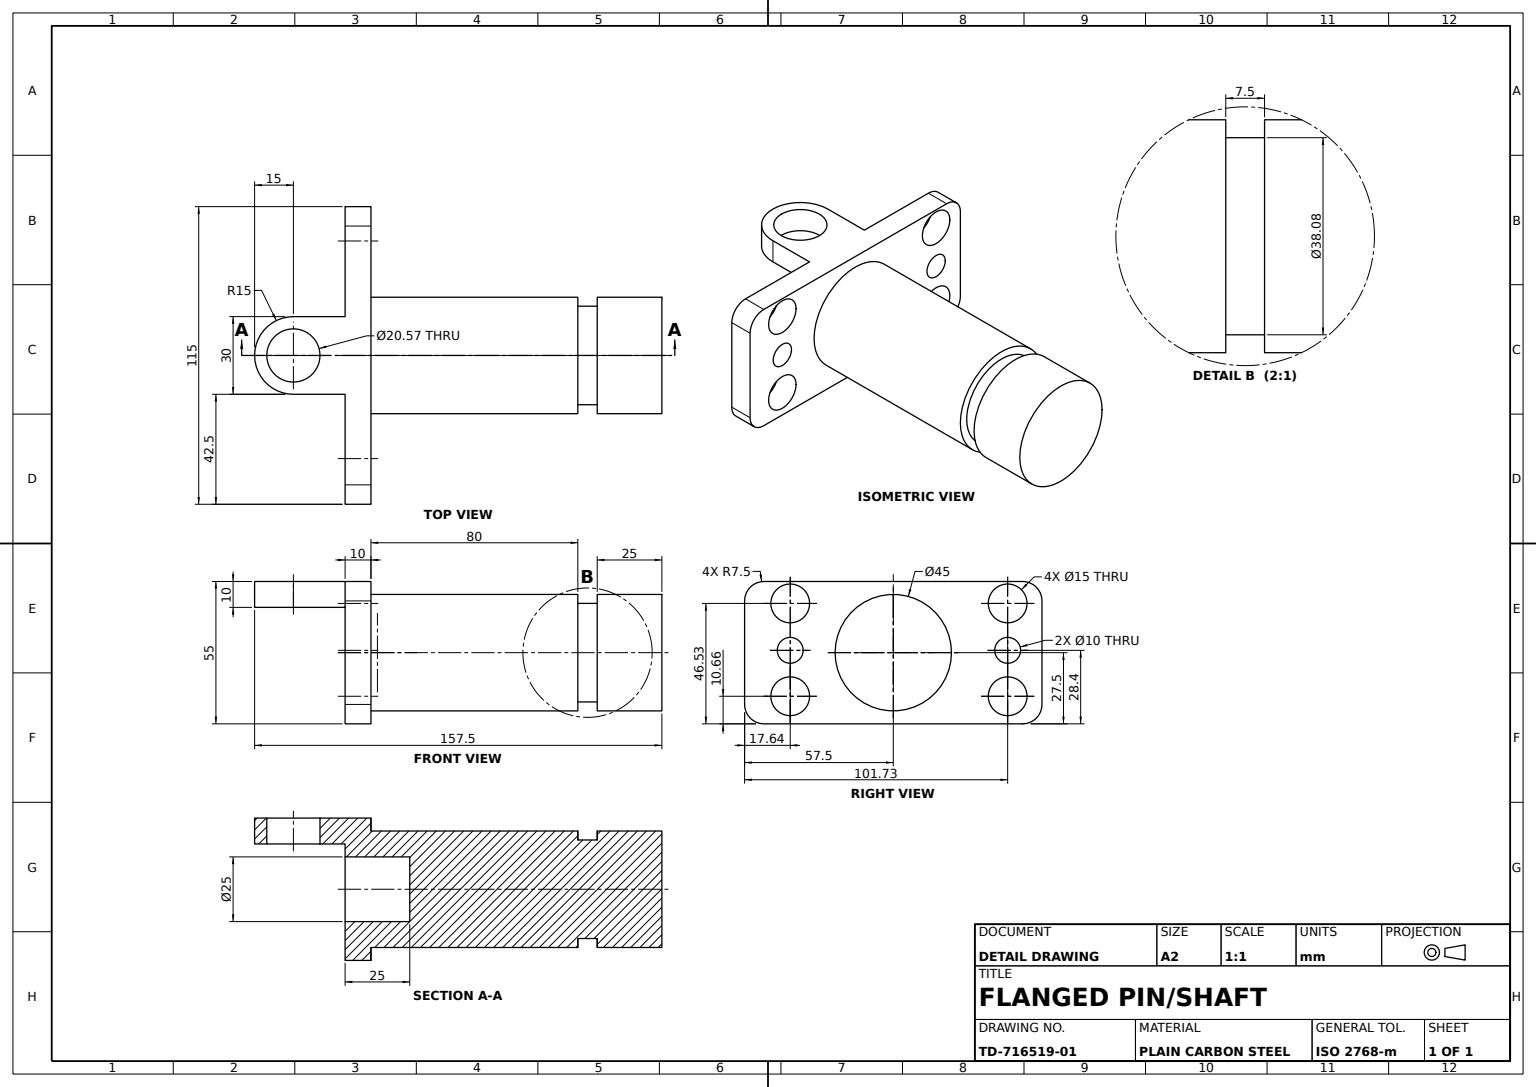
SolidWorks part; units mm, degrees
material "Plain Carbon Steel"
ref_plane "Front Plane" through (0, 0, 0) normal (0, 0, 1) x (1, 0, 0)
ref_plane "Top Plane" through (0, 0, 0) normal (0, 1, 0) x (1, 0, 0)
ref_plane "Right Plane" through (0, 0, 0) normal (1, 0, 0) x (0, 0, -1)
sketch "Flange Plate Sketch" plane through (0, 0, 0) normal (0, 0, 1) x (1, 0, 0)
  line L0 (0, 0) -> (50, 0)
  line L2 (0, 0) -> (-50, 0)
  line L4 (-57.5, 7.5) -> (-57.5, 47.5)
  line L6 (57.5, 7.5) -> (57.5, 47.5)
  line L8 (-50, 55) -> (50, 55)
  arc A0 (50, 0) -> (57.5, 7.5) centre (50, 7.5) ccw
  arc A1 (-57.5, 7.5) -> (-50, 0) centre (-50, 7.5) ccw
  arc A2 (-50, 55) -> (-57.5, 47.5) centre (-50, 47.5) ccw
  arc A3 (57.5, 47.5) -> (50, 55) centre (50, 47.5) ccw
  dimension "D1" = 15
  dimension "D2" = 15
  dimension "D3" = 15
  dimension "D4" = 15
  dimension "D5" = 7.5
  dimension "D6" = 57.5
  dimension "D7" = 55
extrude "Flange Plate" add sketch "Flange Plate Sketch" along normal blind 10
sketch "Shaft Ø45 Sketch" plane through (0, 0, 0) normal (0, 0, -1) x (-1, 0, 0)
  line L0 (57.5, 47.5) -> (57.5, 7.5) construction
  line L1 (50, 0) -> (-50, 0) construction
  circle A0 centre (0, 27.5) radius 22.5
  dimension "D1" = 45
  dimension "D2" = 45
  dimension "D3" = 57.5
  dimension "D4" = 27.5
extrude "Shaft Ø45" add sketch "Shaft Ø45 Sketch" along normal blind 80
sketch "Groove Neck Sketch" plane through (0, 0, -80) normal (0, 0, -1) x (-1, 0, 0)
  circle A0 centre (0, 27.5) radius 19.0386
  dimension "D1" = 38.0771
  dimension "D2" = 38.0771
extrude "Groove Neck Ø38" add sketch "Groove Neck Sketch" along normal blind 7.5
sketch "Shaft End Sketch" plane through (0, 0, -87.5) normal (0, 0, -1) x (-1, 0, 0)
  circle A0 centre (0, 27.5) radius 22.5
  dimension "D1" = 45
  dimension "D2" = 45
extrude "Shaft End Ø45" add sketch "Shaft End Sketch" along normal blind 25
sketch "Centre Bore Sketch" plane through (0, 0, 10) normal (0, 0, 1) x (1, 0, 0)
  line L0 (57.5, 7.5) -> (57.5, 47.5) construction
  line L1 (-50, 0) -> (50, 0) construction
  circle A0 centre (0, 27.5) radius 12.5
  dimension "D1" = 25
  dimension "D2" = 25
  dimension "D3" = 57.5
  dimension "D4" = 27.5
extrude "Centre Bore Ø25" cut sketch "Centre Bore Sketch" against normal blind 25
sketch "Flange Holes Sketch" plane through (0, 0, 10) normal (0, 0, 1) x (1, 0, 0)
  line L0 (57.5, 7.5) -> (57.5, 47.5) construction
  line L1 (-50, 0) -> (50, 0) construction
  circle A0 centre (39.859, 46.5295) radius 7.5
  circle A1 centre (39.859, 28.4) radius 5
  circle A2 centre (39.859, 10.6564) radius 7.5
  circle A3 centre (-44.2306, 10.6564) radius 7.5
  circle A4 centre (-44.2306, 28.4) radius 5
  circle A5 centre (-44.2306, 46.5295) radius 7.5
  dimension "D1" = 15
  dimension "D2" = 10
  dimension "D3" = 15
  dimension "D4" = 15
  dimension "D5" = 10
  dimension "D6" = 15
  dimension "D7" = 10
  dimension "D8" = 15
  dimension "D9" = 17.641
  dimension "D10" = 101.7306
  dimension "D11" = 10.6564
  dimension "D12" = 28.4
  dimension "D13" = 46.5295
extrude "Flange Holes 6x" cut sketch "Flange Holes Sketch" against normal blind 25
sketch "Lug Sketch" plane through (0, 55, 0) normal (0, 1, 0) x (1, 0, 0)
  line L0 (0, -10) -> (-15, -10)
  line L1 (50, -10) -> (-50, -10) construction
  line L2 (-15, -10) -> (-15, -30)
  line L3 (0, -10) -> (15, -10)
  line L4 (15, -10) -> (15, -30)
  line L6 (50, 0) -> (-50, 0) construction
  arc A0 (-15, -30) -> (15, -30) centre (0, -30) ccw
  dimension "D1" = 30
  dimension "D2" = 15
  dimension "D3" = 30
extrude "Lug" add sketch "Lug Sketch" against normal blind 10
sketch "Lug Hole Sketch" plane through (0, 45, 0) normal (0, -1, 0) x (1, 0, 0)
  circle A0 centre (0, 30) radius 10.2867
  dimension "D1" = 20.5734
  dimension "D2" = 20.5734
extrude "Lug Hole Ø20.6" cut sketch "Lug Hole Sketch" against normal blind 10
